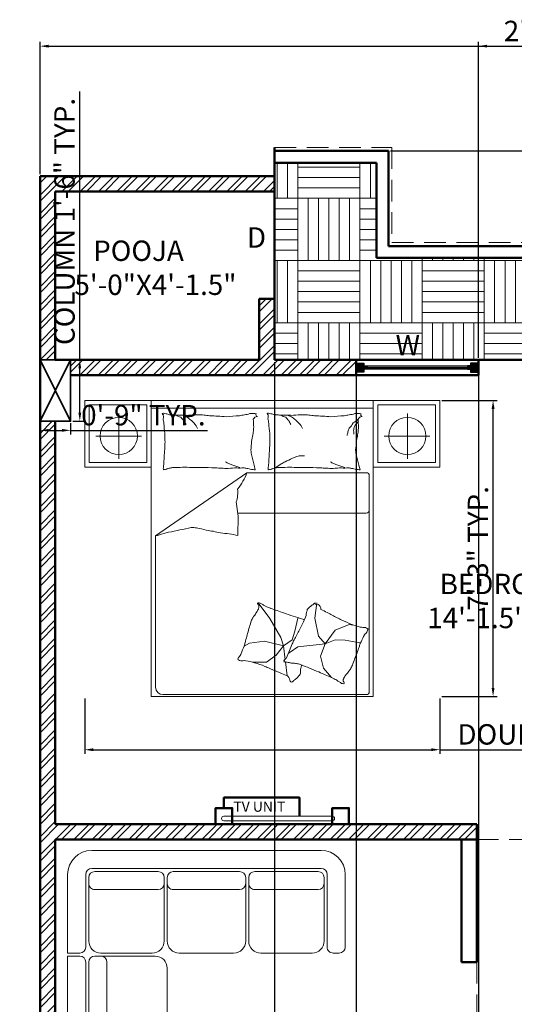
# Model space of a CAD drawing. Units: millimetres. Extents: x 67033 to 68301, y 155969 to 157209.
# Tile 14 of 17: x 67492 to 67638, y 156894 to 157183. Entities that reach past the tile are written whole.
import ezdxf

# ---------------------------------------------------------------- set-up
doc = ezdxf.new("R2010")
doc.units = ezdxf.units.MM
doc.linetypes.add('HIDDEN', pattern=[9.525, 6.35, -3.175])
for name, color, linetype, lineweight in [('A-ANNO-DIMS', 2, 'Continuous', 18), ('A-ANNO-TEXT', 7, 'Continuous', 18), ('A-AREA-IDEN', 3, 'Continuous', 18), ('A-COLS', 3, 'Continuous', 35), ('A-FLOR-OVHD', 1, 'HIDDEN', 18), ('A-FLOR-PATT', 252, 'Continuous', 13), ('A-FURN', 8, 'Continuous', 18), ('A-GLAZ', 4, 'Continuous', 25), ('A-WALL', 7, 'Continuous', 50), ('A-WALL-PATT', 8, 'Continuous', 13)]:
    doc.layers.add(name, color=color, linetype=linetype, lineweight=lineweight)
doc.styles.add('DIM_FONT', font='SIMPLEX.shx', dxfattribs={"width": 0.8})
doc.styles.get("Standard").update_dxf_attribs({"font": 'arial.ttf'})
doc.dimstyles.new('ISO-25', dxfattribs={"dimtxt": 6, "dimasz": 2.5, "dimexe": 1.25, "dimexo": 0.625, "dimtad": 1, "dimdec": 0, "dimlunit": 3, "dimtxsty": 'Standard', "dimcen": 2.5, "dimadec": 0, "dimazin": 0, "dimtfac": 1, "dimtdec": 0, "dimtmove": 0, "dimatfit": 3, "dimfxl": 1, "dimarcsym": 0})
pattern_1 = [(45, (429.8785, 0), (-2.69407684, 2.69407684), []), (45, (431.6745, 0), (-2.69407684, 2.69407684), [])]

# ---------------------------------------------------------------- blocks, each defined once
blk = doc.blocks.new('A$C79766A75')
for p, q in [((0.45, 1.9999), (0, 1.9999)), ((0, 1.9999), (0, 1.5499)), ((0.45, 1.5499), (0.45, 1.9999)), ((1.9506, 2), (0.4506, 2)), ((0.4506, 2), (0.4506, 0)), ((1.9506, 0), (1.9506, 2)), ((2.402, 1.9999), (1.952, 1.9999)), ((1.952, 1.9999), (1.952, 1.5499)), ((2.402, 1.5499), (2.402, 1.9999)), ((0.42, 1.9699), (0.03, 1.9699)), ((0.03, 1.9699), (0.03, 1.5799)), ((0.42, 1.5799), (0.42, 1.9699)), ((1.9506, 1.9476), (0.4506, 1.9476)), ((2.372, 1.9699), (1.982, 1.9699)), ((1.982, 1.9699), (1.982, 1.5799)), ((2.372, 1.5799), (2.372, 1.9699)), ((0.2304, 1.9125), (0.2304, 1.6061)), ((2.1824, 1.9125), (2.1824, 1.6061)), ((0.0743, 1.7595), (0.3834, 1.7595)), ((2.0263, 1.7595), (2.3354, 1.7595)), ((0.4234, 1.6034), (0.4228, 1.6034)), ((1.1461, 1.5617), (1.1254, 1.6443)), ((1.8553, 1.5617), (1.8346, 1.6443)), ((0, 1.5499), (0.45, 1.5499)), ((0.03, 1.5799), (0.42, 1.5799)), ((1.1536, 1.5317), (1.1461, 1.5617)), ((1.8628, 1.5317), (1.8553, 1.5617)), ((1.952, 1.5499), (2.402, 1.5499)), ((1.982, 1.5799), (2.372, 1.5799)), ((1.0972, 1.5115), (0.4791, 1.0841)), ((1.0972, 1.5115), (1.9048, 1.5115)), ((1.9248, 1.4915), (1.9248, 0.0322)), ((1.0383, 1.2184), (1.0246, 1.3138)), ((1.9048, 1.2389), (1.0354, 1.2389)), ((1.0365, 1.0883), (1.0383, 1.2184)), ((0.4791, 0.0622), (0.4791, 1.0841)), ((1.1731, 0.6316), (1.2523, 0.5276)), ((1.5696, 0.6317), (1.5559, 0.5286)), ((1.2523, 0.5276), (1.3274, 0.3973)), ((1.4223, 0.4407), (1.442, 0.5296)), ((1.5559, 0.5286), (1.5817, 0.4065)), ((1.6952, 0.4478), (1.7898, 0.4856)), ((1.7898, 0.4856), (1.8139, 0.4822)), ((1.4025, 0.3834), (1.4223, 0.4407)), ((1.5817, 0.4065), (1.6264, 0.355)), ((1.6264, 0.355), (1.6952, 0.4478)), ((1.1139, 0.3597), (1.0779, 0.3397)), ((1.2167, 0.3736), (1.1139, 0.3597)), ((1.3452, 0.342), (1.2167, 0.3736)), ((1.2957, 0.2787), (1.3452, 0.342)), ((1.3274, 0.3973), (1.3452, 0.342)), ((1.3452, 0.342), (1.4025, 0.3834)), ((1.3452, 0.342), (1.3569, 0.2478)), ((1.4034, 0.3558), (1.3803, 0.2995)), ((1.4406, 0.3361), (1.3907, 0.3)), ((1.6264, 0.355), (1.4406, 0.3361)), ((1.5954, 0.2725), (1.6264, 0.355)), ((1.6264, 0.355), (1.6935, 0.3825)), ((1.6935, 0.3825), (1.7623, 0.379)), ((1.7623, 0.379), (1.8603, 0.3619)), ((1.8603, 0.3619), (1.8636, 0.3554)), ((1.2305, 0.2313), (1.2957, 0.2787)), ((1.3803, 0.2995), (1.3626, 0.256)), ((1.3907, 0.3), (1.3787, 0.2914)), ((1.6161, 0.19), (1.5954, 0.2725)), ((1.1376, 0.2313), (1.2305, 0.2313)), ((1.3588, 0.2331), (1.3706, 0.1385)), ((1.6697, 0.1274), (1.6161, 0.19)), ((1.9048, 0.0122), (0.5291, 0.0122)), ((0.4506, 0), (1.9506, 0))]:
    blk.add_line(p, q)
for centre in [(0.2304, 1.7595), (2.1824, 1.7595)]:
    blk.add_circle(centre, 0.126)
for centre, radius, start, end in [((0.5232, 1.9139), 0.00342, 291.7883, 340.43603), ((0.525, 1.9085), 0.00232, 340.43603, 101.89306), ((0.5246, 1.9378), 0.0251, 274.30254, 291.7883), ((0.5311, 1.9093), 0.00428, 201.9904, 281.89306), ((0.4996, 1.8889), 0.0328, 338.57902, 8.13348), ((0.2896, 1.8253), 0.246, 8.13348, 12.10946), ((0.5465, 1.8994), 0.0156, 158.57902, 201.9904), ((0.5486, 1.9393), 0.0289, 239.34875, 274.30254), ((0.5458, 1.8568), 0.0539, 59.34875, 84.74081), ((0.546, 1.0829), 0.8208, 84.74081, 88.09211), ((0.6118, 2.0005), 0.0992, 254.06476, 274.21588), ((0.6775, 1.9817), 0.0992, 233.91364, 254.06476), ((0.6362, 0.406), 1.4943, 88.09211, 90.57574), ((0.7304, 1.9449), 0.0992, 216.17665, 233.91364), ((0.7737, 2.1075), 0.234, 242.76041, 249.13972), ((0.7661, 1.8961), 0.0992, 198.43965, 216.17665), ((0.7591, 1.0293), 0.8732, 90.57574, 94.80185), ((0.738, 1.949), 0.0768, 231.61143, 242.76041), ((0.974, 2.1633), 0.3916, 226.18849, 231.61143), ((0.7631, 2.1919), 0.2897, 267.46141, 274.80185), ((0.8143, 2.0532), 0.1524, 259.81012, 267.46141), ((0.7515, 1.3747), 0.5293, 79.81012, 83.9133), ((0.8451, 0.8466), 1.049, 83.9133, 90), ((1.046, 1.2129), 0.6827, 90, 97.54685), ((1.1117, 1.6625), 0.2422, 97.54685, 105.74398), ((1.0352, 2.2041), 0.3048, 278.43719, 285.74398), ((1.1179, 2.0719), 0.1611, 270, 278.43719), ((1.171, 1.8579), 0.0342, 94.40021, 153.41948), ((1.6324, 1.8735), 0.4918, 180, 186.23236), ((1.1592, 2.0011), 0.0904, 258.72762, 270), ((1.1709, 1.9049), 0.0131, 153.41948, 258.72762), ((1.2325, 1.9139), 0.00342, 291.7883, 340.43603), ((1.2342, 1.9085), 0.00232, 340.43603, 101.89306), ((1.2338, 1.9378), 0.0251, 274.30254, 291.7883), ((1.2404, 1.9093), 0.00428, 201.9904, 281.89306), ((1.2088, 1.8889), 0.0328, 338.57902, 8.13348), ((0.9988, 1.8253), 0.246, 8.13348, 12.10946), ((1.2558, 1.8994), 0.0156, 158.57902, 201.9904), ((1.2578, 1.9393), 0.0289, 239.34875, 274.30254), ((1.2551, 1.8568), 0.0539, 59.34875, 84.74081), ((1.2552, 1.0829), 0.8208, 84.74081, 88.09211), ((1.3211, 2.0005), 0.0992, 254.06476, 274.21588), ((1.3868, 1.9817), 0.0992, 233.91364, 254.06476), ((1.3455, 0.406), 1.4943, 88.09211, 90.57574), ((1.4396, 1.9449), 0.0992, 216.17665, 233.91364), ((1.4829, 2.1075), 0.234, 242.76041, 249.13972), ((1.4753, 1.8961), 0.0992, 198.43965, 216.17665), ((1.4683, 1.0293), 0.8732, 90.57574, 94.80185), ((1.4473, 1.949), 0.0768, 231.61143, 242.76041), ((1.6833, 2.1633), 0.3916, 226.18849, 231.61143), ((1.4724, 2.1919), 0.2897, 267.46141, 274.80185), ((1.5236, 2.0532), 0.1524, 259.81012, 267.46141), ((1.4607, 1.3747), 0.5293, 79.81012, 83.9133), ((1.5543, 0.8466), 1.049, 83.9133, 90), ((1.7552, 1.2129), 0.6827, 90, 97.54685), ((1.821, 1.6625), 0.2422, 97.54685, 105.74398), ((1.7444, 2.2041), 0.3048, 278.43719, 285.74398), ((1.7511, 1.9723), 0.1399, 297.20359, 314.90238), ((1.8271, 2.0719), 0.1611, 270, 278.43719), ((1.8802, 1.8579), 0.0342, 94.40021, 153.41948), ((2.3416, 1.8735), 0.4918, 180, 186.23236), ((1.8684, 2.0011), 0.0904, 258.72762, 270), ((1.8802, 1.9049), 0.0131, 153.41948, 258.72762), ((0.7297, 1.8867), 0.1983, 187.6809, 192.10946), ((1.4472, 1.8987), 0.9131, 183.36875, 187.6809), ((0.9057, 1.9982), 0.2252, 219.03494, 226.18849), ((0.7932, 1.8591), 0.0493, 208.31676, 219.03494), ((0.9392, 1.9062), 0.2002, 203.00277, 208.31676), ((1.3446, 1.7858), 0.204, 170.31563, 180), ((1.4389, 1.8867), 0.1983, 187.6809, 192.10946), ((2.1565, 1.8987), 0.9131, 183.36875, 187.6809), ((1.615, 1.9982), 0.2252, 219.03494, 226.18849), ((1.5025, 1.8591), 0.0493, 208.31676, 219.03494), ((1.6484, 1.9062), 0.2002, 203.00277, 208.31676), ((1.6554, 1.8529), 0.1399, 332.60117, 343.48502), ((1.6908, 1.9123), 0.1399, 314.90238, 332.60117), ((1.7653, 1.8132), 0.0562, 341.2201, 0), ((1.6307, 1.8895), 0.2056, 338.18508, 341.2201), ((1.6887, 1.8881), 0.1511, 334.64488, 338.18508), ((1.7896, 1.8667), 0.0526, 318.55709, 334.64488), ((1.784, 1.9167), 0.0899, 306.26407, 318.55709), ((2.0538, 1.7858), 0.204, 170.31563, 180), ((1.2208, 1.7573), 0.6787, 178.36691, 183.36875), ((0.8192, 1.792), 0.3171, 347.80162, 351.99495), ((2.0027, 1.5994), 0.882, 167.80162, 170.31563), ((1.9301, 1.7573), 0.6787, 178.36691, 183.36875), ((1.6404, 1.8023), 0.1399, 343.48502, 354.36887), ((1.73, 1.7719), 0.0915, 0, 14.68511), ((1.5284, 1.792), 0.3171, 347.80162, 351.99495), ((2.7119, 1.5994), 0.882, 167.80162, 170.31563), ((14.1519, 0.85), 13.6356, 176.49514, 176.94504), ((1.9066, 1.6447), 1.3652, 176.94504, 178.36691), ((0.4711, 1.7556), 0.6588, 351.99495, 357.33512), ((1.0578, 1.6474), 0.0677, 357.33512, 14.04519), ((14.8612, 0.85), 13.6356, 176.49514, 176.94504), ((2.6158, 1.6447), 1.3652, 176.94504, 178.36691), ((1.1803, 1.7556), 0.6588, 351.99495, 357.33512), ((1.767, 1.6474), 0.0677, 357.33512, 14.04519), ((0.7658, 2.8912), 1.4323, 294.32653, 296.49848), ((1.226, 2.0834), 0.5066, 290.67428, 294.32653), ((1.4305, 1.6796), 0.058, 274.08277, 290.67428), ((1.4679, 1.8969), 0.2721, 266.4448, 274.08277), ((0.8521, 1.5209), 0.3212, 170.00164, 176.49514), ((0.513, 1.535), 0.0193, 350.00164, 16.69777), ((0.5322, 1.5304), 0.00132, 16.69777, 97.12039), ((0.5579, 1.4467), 0.0875, 97.12039, 106.22115), ((0.5822, 1.4654), 0.0767, 106.22115, 117.28412), ((0.5507, 1.5832), 0.0453, 282.86904, 297.28412), ((0.5623, 1.6885), 0.1459, 273.57397, 282.86904), ((0.589, 2.7103), 1.164, 270.28654, 273.57397), ((0.7584, 7.2662), 5.7185, 269.02962, 270.28654), ((0.9401, 4.9065), 3.3622, 267.39037, 269.02962), ((0.9811, 2.7573), 1.2165, 265.38242, 267.39037), ((0.8583, 0.139), 1.4048, 85.38242, 87.25094), ((0.6583, 0.9067), 0.7387, 64.68893, 66.51559), ((1.0175, 1.3138), 0.2301, 87.25094, 101.55856), ((0.7015, 0.888), 0.7387, 66.51559, 68.34226), ((0.7501, 0.8688), 0.7387, 68.34226, 70.57202), ((0.8043, 0.8497), 0.7387, 70.57202, 72.80178), ((1.0449, 1.6886), 0.1459, 263.56595, 281.55856), ((1.1099, 1.6599), 0.1197, 252.61359, 263.56595), ((1.0587, 1.3144), 0.2297, 72.61359, 80.5159), ((1.108, 1.2635), 0.2708, 80.5159, 85.91706), ((1.1535, 1.5308), 0.000917, 85.91706, 194.04494), ((1.5613, 1.5209), 0.3212, 170.00164, 176.49514), ((1.2222, 1.535), 0.0193, 350.00164, 16.69777), ((1.2414, 1.5304), 0.00132, 16.69777, 97.12039), ((1.2671, 1.4467), 0.0875, 97.12039, 106.22115), ((1.2914, 1.4654), 0.0767, 106.22115, 117.28412), ((1.2599, 1.5832), 0.0453, 282.86904, 297.28412), ((1.2716, 1.6885), 0.1459, 273.57397, 282.86904), ((0.9025, 2.1618), 0.7286, 302.13498, 305.82629), ((1.2982, 2.7103), 1.164, 270.28654, 273.57397), ((1.1895, 1.8508), 0.3126, 296.49848, 302.13498), ((1.4677, 7.2662), 5.7185, 269.02962, 270.28654), ((1.6493, 4.9065), 3.3622, 267.39037, 269.02962), ((1.6903, 2.7573), 1.2165, 265.38242, 267.39037), ((1.5676, 0.139), 1.4048, 85.38242, 87.25094), ((1.3675, 0.9067), 0.7387, 64.68893, 66.51559), ((1.7268, 1.3138), 0.2301, 87.25094, 101.55856), ((1.4107, 0.888), 0.7387, 66.51559, 68.34226), ((1.4594, 0.8688), 0.7387, 68.34226, 70.57202), ((1.5136, 0.8497), 0.7387, 70.57202, 72.80178), ((1.7541, 1.6886), 0.1459, 263.56595, 281.55856), ((1.8192, 1.6599), 0.1197, 252.61359, 263.56595), ((1.7679, 1.3144), 0.2297, 72.61359, 80.5159), ((1.8172, 1.2635), 0.2708, 80.5159, 85.91706), ((1.8627, 1.5308), 0.000917, 85.91706, 194.04494), ((0.745, 1.6407), 0.3751, 320.35546, 339.85116), ((1.9048, 1.4915), 0.02, 0, 90), ((0.8556, 1.3759), 0.1801, 339.85116, 8.13558), ((1.9048, 1.2589), 0.02, 270, 0), ((-0.1888, 5.1029), 4.0646, 280.72756, 282.92554), ((0.7282, 1.1989), 0.0581, 262.26962, 280.72756), ((0.7833, 1.3309), 0.1942, 256.8096, 262.26962), ((0.2481, -1.3253), 2.5158, 76.8096, 78.32586), ((-0.0248, 2.8487), 1.8351, 285.93519, 287.73639), ((0.3872, 1.7415), 0.6574, 282.92554, 285.93519), ((0.3953, -1.4284), 2.588, 78.32586, 80.50498), ((0.413, -2.64), 3.7801, 80.50498, 82.308), ((1.1752, 0.6267), 0.0063, 166.71916, 233.42082), ((1.1734, 0.6272), 0.00443, 93.94836, 166.71916), ((1.163, 0.6103), 0.0142, 10.40739, 53.42082), ((1.1755, 0.5964), 0.0352, 69.65479, 93.94836), ((1.1011, 0.5989), 0.0771, 2.72862, 10.40739), ((1.1628, 0.6019), 0.0153, 345.42909, 2.72862), ((1.1669, 0.5731), 0.0601, 51.41461, 69.65479), ((1.2538, 0.682), 0.0792, 231.41461, 247.29308), ((1.5463, 1.3811), 0.8371, 247.29308, 249.87133), ((1.383, 0.7705), 0.2176, 307.21509, 313.52244), ((1.1426, 1.1456), 0.6605, 306.2163, 307.21509), ((1.7751, 0.3162), 0.3825, 126.2163, 127.52874), ((1.5806, 0.5924), 0.0452, 127.52874, 134.1274), ((1.5093, 0.6825), 0.0697, 308.81361, 314.1274), ((1.5706, 0.6318), 0.0127, 176.75451, 308.81361), ((1.5621, 0.59), 0.0359, 356.75451, 62.70976), ((1.2077, 0.4922), 0.081, 140.29953, 153.92651), ((0.9961, 0.6678), 0.194, 320.29953, 329.09437), ((0.8605, 0.749), 0.352, 329.09437, 333.18207), ((1.1396, 0.6079), 0.0393, 333.18207, 345.42909), ((3.0113, 5.3783), 5.0942, 249.87133, 250.91638), ((2.374, 3.5362), 3.145, 250.91638, 253.39153), ((2.4089, 0.1204), 1.0054, 154.94715, 157.58378), ((1.5435, 0.5526), 0.0458, 157.58378, 188.04918), ((1.4828, 0.5833), 0.0226, 324.10643, 8.04918), ((1.4519, 0.6426), 0.0774, 313.52244, 324.10643), ((0.2201, -2.1858), 3.0972, 62.70976, 63.58535), ((2.5711, 2.3551), 2.0162, 242.50014, 243.58535), ((4.5245, 5.9445), 6.1019, 242.15178, 242.50014), ((3.0311, -0.112), 2.003, 162.1604, 164.73746), ((1.3115, 0.4414), 0.1965, 153.92651, 162.1604), ((2.9813, -0.2643), 1.6868, 152.91165, 154.94715), ((1.5084, 0.6341), 0.1166, 253.39153, 259.26338), ((-0.9881, -4.647), 5.8383, 62.15178, 62.50792), ((1.5182, -0.068), 0.6236, 62.50792, 69.25137), ((1.7121, 0.0657), 0.43, 69.25137, 77.37478), ((1.8682, 0.4049), 0.063, 77.37478, 93.38812), ((1.8955, 0.5247), 0.0599, 256.95977, 273.38812), ((2.6887, -0.0186), 1.6481, 164.73746, 166.159), ((2.8096, -0.3311), 1.5652, 150.06403, 152.91165), ((-0.5166, 1.5491), 2.6619, 333.66682, 334.82685), ((1.8435, 0.4743), 0.0755, 310.50865, 333.66682), ((1.9257, 0.5082), 0.0509, 238.30826, 256.95977), ((1.9279, 0.441), 0.0168, 130.50865, 180.96136), ((1.9201, 0.4587), 0.0058, 180.96136, 238.30826), ((-1.4109, 1.284), 2.6619, 338.0627, 339.22273), ((0.9098, 0.4035), 0.1798, 339.22273, 343.68776), ((0.5589, 0.5062), 0.5454, 343.68776, 346.159), ((1.2176, 0.4627), 0.2143, 330.06403, 337.76452), ((3.4079, -0.2212), 1.6481, 160.34158, 161.76311), ((1.3456, 0.5261), 0.5454, 339.29188, 341.76311), ((1.701, 0.4319), 0.1798, 334.82685, 339.29188), ((0.9882, 0.3177), 0.0755, 314.90453, 338.0627), ((3.6966, -0.4634), 2.003, 157.76452, 160.34158), ((1.0533, 0.2524), 0.0168, 134.90453, 185.35724), ((1.0424, 0.2513), 0.0058, 185.35724, 242.70414), ((1.0631, 0.2914), 0.0509, 242.70414, 261.35565), ((1.0645, 0.3003), 0.0599, 261.35565, 277.784), ((1.0811, 0.1786), 0.063, 81.77066, 97.784), ((1.0286, -0.1846), 0.43, 73.64725, 81.77066), ((0.974, -0.3705), 0.6236, 66.9038, 73.64725), ((-1.0716, -5.1672), 5.8383, 66.54766, 66.9038), ((1.3465, 0.2383), 0.00467, 287.18674, 70.62007), ((1.3486, 0.2247), 0.0092, 70.62007, 94.25932), ((1.3694, 0.234), 0.0231, 107.18674, 157.76452), ((1.3563, 0.267), 0.034, 262.01776, 274.25932), ((1.4091, 0.4221), 0.1955, 255.1193, 262.01776), ((1.358, 0.0507), 0.1794, 75.1193, 82.32164), ((1.4096, 0.153), 0.0712, 82.32164, 94.51184), ((1.4285, 0.2893), 0.0663, 261.87843, 274.51184), ((1.4755, 0.332), 0.1166, 248.99565, 261.87843), ((2.7121, 3.1012), 3.145, 246.5205, 248.99565), ((2.4175, -0.1202), 1.0054, 160.65521, 161.97966), ((1.9797, 0.1108), 0.1965, 149.53063, 157.76452), ((3.6805, 5.7866), 6.1019, 246.54766, 246.89602), ((2.0773, 2.0287), 2.0162, 246.89602, 247.98123), ((0.1602, -2.7118), 3.0972, 67.10564, 67.98123), ((1.3512, 0.1084), 0.0359, 1.15039, 67.10564), ((1.2874, 0.2845), 0.2176, 311.61098, 317.91833), ((1.3914, 0.1905), 0.0774, 317.91833, 328.50231), ((1.4382, 0.1619), 0.0226, 328.50231, 12.44506), ((1.505, 0.1766), 0.0458, 161.97966, 192.44506), ((3.6993, 4.7998), 5.0942, 245.47545, 246.5205), ((1.4661, 0.3294), 0.352, 324.69849, 328.78619), ((1.6279, 0.2819), 0.194, 315.90365, 324.69849), ((1.856, 0.1288), 0.081, 135.90365, 149.53063), ((1.3997, 0.1094), 0.0127, 181.15039, 313.2095), ((1.3607, 0.1509), 0.0697, 313.2095, 318.52329), ((1.4468, 0.0748), 0.0452, 131.92462, 138.52329), ((1.6722, -0.1762), 0.3825, 130.61218, 131.92462), ((0.9933, 0.6156), 0.6605, 310.61218, 311.61098), ((2.051, 0.8725), 0.8371, 242.8972, 245.47545), ((1.7576, 0.1689), 0.0792, 227.01873, 242.8972), ((1.6963, 0.0438), 0.0601, 47.01873, 65.25891), ((1.737, 0.0526), 0.0352, 65.25891, 89.55248), ((1.7345, 0.1188), 0.0153, 341.03321, 358.33274), ((1.6723, 0.1058), 0.0771, 358.33274, 6.01151), ((1.7401, 0.0928), 0.0142, 6.01151, 49.02494), ((1.7162, 0.1388), 0.0393, 328.78619, 341.03321), ((1.756, 0.0832), 0.00443, 89.55248, 162.32327), ((1.7602, 0.0924), 0.0063, 162.32327, 229.02494), ((0.5291, 0.0622), 0.05, 180, 270), ((1.9048, 0.0322), 0.02, 270, 0)]:
    blk.add_arc(centre, radius, start, end)
at = {"style": 'DIM_FONT', "text_generation_flag": 4, "width": 0.8, "flags": 9}
for tag in ['XSIZE', 'YSIZE']:
    blk.add_attdef(tag, (1.9506, 2), '', height=0.0005, rotation=180, dxfattribs=at)
blk = doc.blocks.new('A$C2AFA021D')
for p, q in [((0.8, 2.3), (0.2, 2.3)), ((0.85, 2.2), (0.85, 2.25)), ((0.2, 2.15), (0.8, 2.15)), ((0.225, 2.125), (0.275, 2.125)), ((0.75, 2.125), (0.275, 2.125)), ((0, 2.1), (0, 0.2)), ((0.15, 0.2), (0.15, 2.1)), ((0.175, 1.55), (0.175, 2.075)), ((0.325, 2.075), (0.325, 1.55)), ((0.85, 1.6), (0.85, 2.025)), ((0.275, 1.5), (0.225, 1.5)), ((0.225, 1.475), (0.275, 1.475)), ((0.275, 1.5), (0.75, 1.5)), ((0.75, 1.475), (0.275, 1.475)), ((0.175, 0.875), (0.175, 1.425)), ((0.325, 1.425), (0.325, 0.875)), ((0.85, 0.925), (0.85, 1.375)), ((0.275, 0.825), (0.225, 0.825)), ((0.275, 0.825), (0.75, 0.825)), ((0.975, 0.825), (1.4, 0.825)), ((1.625, 0.825), (2.075, 0.825)), ((2.3, 0.825), (2.725, 0.825)), ((2.9, 0.825), (2.95, 0.825)), ((0.175, 0.225), (0.175, 0.75)), ((0.225, 0.8), (0.275, 0.8)), ((0.75, 0.8), (0.275, 0.8)), ((0.325, 0.75), (0.325, 0.225)), ((2.85, 0.2), (2.85, 0.775)), ((3, 0.775), (3, 0.2)), ((0.85, 0.275), (0.85, 0.7)), ((0.875, 0.275), (0.875, 0.725)), ((1.5, 0.725), (1.5, 0.275)), ((1.525, 0.275), (1.525, 0.725)), ((2.175, 0.725), (2.175, 0.275)), ((2.2, 0.275), (2.2, 0.725)), ((2.825, 0.725), (2.825, 0.275)), ((0.875, 0.275), (0.875, 0.225)), ((1.45, 0.325), (0.925, 0.325)), ((1.5, 0.225), (1.5, 0.275)), ((1.525, 0.275), (1.525, 0.225)), ((2.125, 0.325), (1.575, 0.325)), ((2.175, 0.225), (2.175, 0.275)), ((2.2, 0.275), (2.2, 0.225)), ((2.775, 0.325), (2.25, 0.325)), ((2.825, 0.225), (2.825, 0.275)), ((0.275, 0.175), (0.225, 0.175)), ((0.275, 0.175), (0.75, 0.175)), ((0.925, 0.175), (1.45, 0.175)), ((1.575, 0.175), (2.125, 0.175)), ((2.25, 0.175), (2.775, 0.175)), ((0.8, 0.15), (0.2, 0.15)), ((0.85, 0), (0.85, 0.1)), ((0.875, 0.1), (0.875, 0)), ((0.925, 0.15), (2.8, 0.15)), ((0.2, 0), (0.85, 0)), ((2.8, 0), (0.875, 0))]:
    blk.add_line(p, q)
for centre, radius, start, end in [((0.2, 2.1), 0.2, 90, 180), ((0.8, 2.25), 0.05, 0, 90), ((0.2, 2.1), 0.05, 90, 180), ((0.225, 2.075), 0.05, 90, 180), ((0.275, 2.075), 0.05, 0, 90), ((0.75, 2.025), 0.1, 0, 90), ((0.8, 2.2), 0.05, 270, 0), ((0.225, 1.55), 0.05, 180, 270), ((0.275, 1.55), 0.05, 270, 0), ((0.75, 1.6), 0.1, 270, 0), ((0.225, 1.425), 0.05, 90, 180), ((0.275, 1.425), 0.05, 0, 90), ((0.75, 1.375), 0.1, 360, 90), ((0.75, 0.925), 0.1, 270, 0), ((0.225, 0.875), 0.05, 180, 270), ((0.275, 0.875), 0.05, 270, 0), ((0.975, 0.725), 0.1, 90, 180), ((1.4, 0.725), 0.1, 0, 90), ((1.625, 0.725), 0.1, 90, 180), ((2.075, 0.725), 0.1, 0, 90), ((2.3, 0.725), 0.1, 90, 180), ((2.725, 0.725), 0.1, 0, 90), ((2.9, 0.775), 0.05, 90, 180), ((2.95, 0.775), 0.05, 0, 90), ((0.225, 0.75), 0.05, 90, 180), ((0.275, 0.75), 0.05, 0, 90), ((0.75, 0.7), 0.1, 0, 90), ((0.75, 0.275), 0.1, 270, 0), ((0.925, 0.275), 0.05, 90, 180), ((1.45, 0.275), 0.05, 360, 90), ((1.575, 0.275), 0.05, 90, 180), ((2.125, 0.275), 0.05, 360, 90), ((2.25, 0.275), 0.05, 90, 180), ((2.775, 0.275), 0.05, 360, 90), ((0.2, 0.2), 0.2, 180, 270), ((0.2, 0.2), 0.05, 180, 270), ((0.225, 0.225), 0.05, 180, 270), ((0.275, 0.225), 0.05, 270, 0), ((0.925, 0.225), 0.05, 180, 270), ((1.45, 0.225), 0.05, 270, 0), ((1.575, 0.225), 0.05, 180, 270), ((2.125, 0.225), 0.05, 270, 0), ((2.25, 0.225), 0.05, 180, 270), ((2.775, 0.225), 0.05, 270, 0), ((2.8, 0.2), 0.2, 270, 0), ((2.8, 0.2), 0.05, 270, 0), ((0.8, 0.1), 0.05, 0, 90), ((0.925, 0.1), 0.05, 90, 180)]:
    blk.add_arc(centre, radius, start, end)
blk = doc.blocks.new('WIN-900')
for p, q in [((3.67, 3.22), (33.2, 3.22)), ((3.67, 2.74), (33.2, 2.74)), ((33.2, 2.27), (3.67, 2.27))]:
    blk.add_line(p, q)
blk.add_lwpolyline([(0.44, 4.99), (36.44, 4.99), (36.44, 0.49), (0.44, 0.49)], close=True)
for points in [[(0.44, 4.09), (2.73, 4.09), (2.73, 3.22), (3.67, 3.22), (3.67, 2.27), (2.73, 2.27), (2.73, 1.4), (0.44, 1.4)], [(36.44, 4.09), (34.14, 4.09), (34.14, 3.22), (33.2, 3.22), (33.2, 2.27), (34.14, 2.27), (34.14, 1.4), (36.44, 1.4)]]:
    blk.add_lwpolyline(points)
blk = doc.blocks.new('COLUMN-230x460')
for p, q in [((0.44, 17.99), (9.44, -0.01)), ((9.44, 17.99), (0.44, -0.01))]:
    blk.add_line(p, q)
blk.add_lwpolyline([(0.44, 17.99), (9.44, 17.99), (9.44, -0.01), (0.44, -0.01)], close=True)
blk = doc.blocks.new('TV-UNIT')
for points in [[(0.68, 1.36), (32.57, 1.36)], [(32.57, 0), (0.68, 0)]]:
    blk.add_lwpolyline(points)
for centre, start, end in [((0.68, 0.68), 90, 270), ((32.57, 0.68), 270, 90)]:
    blk.add_arc(centre, 0.678, start, end)
blk = doc.blocks.new('*D49')
at = {"layer": 'A-ANNO-DIMS', "color": 0, "lineweight": -2, "transparency": 16777216}
for p, q in [((67510.02, 157082.99), (67510.02, 157161.9)), ((67507.94, 157082.99), (67511.27, 157082.99)), ((67510.02, 157067.49), (67510.02, 157080.49)), ((67507.94, 157064.99), (67511.27, 157064.99))]:
    blk.add_line(p, q, dxfattribs=at)
at = {"layer": 'A-ANNO-DIMS', "color": 0, "transparency": 16777216}
for points in [[(67509.6, 157080.49), (67510.43, 157080.49), (67510.02, 157082.99)], [(67509.6, 157067.49), (67510.43, 157067.49), (67510.02, 157064.99)]]:
    blk.add_solid(points, dxfattribs=at)
at = {"layer": 'Defpoints', "color": 0, "transparency": 16777216}
for p in [(67507.32, 157082.99), (67510.02, 157082.99), (67507.32, 157064.99)]:
    blk.add_point(p, dxfattribs=at)
at = {"layer": 'A-ANNO-DIMS', "color": 0, "transparency": 16777216, "insert": (67506.29, 157123.7), "char_height": 6, "attachment_point": 5, "rotation": 90}
blk.add_mtext('COLUMN 1\'-6" TYP.', dxfattribs=at)
blk = doc.blocks.new('*D50')
at = {"layer": 'A-ANNO-DIMS', "color": 0, "lineweight": -2, "transparency": 16777216}
for p, q in [((67498.32, 157064.37), (67498.32, 157061.04)), ((67507.32, 157064.37), (67507.32, 157061.04)), ((67500.82, 157062.29), (67504.82, 157062.29)), ((67507.32, 157062.29), (67547.64, 157062.29))]:
    blk.add_line(p, q, dxfattribs=at)
at = {"layer": 'A-ANNO-DIMS', "color": 0, "transparency": 16777216}
for points in [[(67500.82, 157062.71), (67500.82, 157061.88), (67498.32, 157062.29)], [(67504.82, 157062.71), (67504.82, 157061.88), (67507.32, 157062.29)]]:
    blk.add_solid(points, dxfattribs=at)
at = {"layer": 'Defpoints', "color": 0, "transparency": 16777216}
for p in [(67498.32, 157064.99), (67507.32, 157064.99), (67507.32, 157062.29)]:
    blk.add_point(p, dxfattribs=at)
at = {"layer": 'A-ANNO-DIMS', "color": 0, "transparency": 16777216, "insert": (67528.73, 157065.98), "char_height": 6, "attachment_point": 5}
blk.add_mtext('0\'-9" TYP.', dxfattribs=at)
blk = doc.blocks.new('*D55')
at = {"layer": 'A-ANNO-DIMS', "color": 0, "lineweight": -2, "transparency": 16777216}
for p, q in [((67511.46, 156983.46), (67511.46, 156967.16)), ((67615.96, 156983.46), (67615.96, 156967.16)), ((67513.96, 156968.41), (67613.46, 156968.41)), ((67615.96, 156968.41), (67726.32, 156968.41))]:
    blk.add_line(p, q, dxfattribs=at)
at = {"layer": 'A-ANNO-DIMS', "color": 0, "transparency": 16777216}
for points in [[(67513.96, 156968.83), (67513.96, 156967.99), (67511.46, 156968.41)], [(67613.46, 156968.83), (67613.46, 156967.99), (67615.96, 156968.41)]]:
    blk.add_solid(points, dxfattribs=at)
at = {"layer": 'Defpoints', "color": 0, "transparency": 16777216}
for p in [(67511.46, 156984.08), (67615.96, 156984.08), (67615.96, 156968.41)]:
    blk.add_point(p, dxfattribs=at)
at = {"layer": 'A-ANNO-DIMS', "color": 0, "transparency": 16777216, "insert": (67672.39, 156972.14), "char_height": 6, "attachment_point": 5}
blk.add_mtext('DOUBLE BED 8\'-8 1/2" TYP.', dxfattribs=at)
blk = doc.blocks.new('*D56')
at = {"layer": 'A-ANNO-DIMS', "color": 0, "lineweight": -2, "transparency": 16777216}
for p, q in [((67616.58, 157071.11), (67632.88, 157071.11)), ((67631.63, 156986.58), (67631.63, 157068.61)), ((67616.58, 156984.08), (67632.88, 156984.08))]:
    blk.add_line(p, q, dxfattribs=at)
at = {"layer": 'A-ANNO-DIMS', "color": 0, "transparency": 16777216}
for points in [[(67631.21, 157068.61), (67632.05, 157068.61), (67631.63, 157071.11)], [(67631.21, 156986.58), (67632.05, 156986.58), (67631.63, 156984.08)]]:
    blk.add_solid(points, dxfattribs=at)
at = {"layer": 'Defpoints', "color": 0, "transparency": 16777216}
for p in [(67615.96, 157071.11), (67631.63, 157071.11), (67615.96, 156984.08)]:
    blk.add_point(p, dxfattribs=at)
at = {"layer": 'A-ANNO-DIMS', "color": 0, "transparency": 16777216, "insert": (67627.94, 157027.6), "char_height": 6, "attachment_point": 5, "rotation": 90}
blk.add_mtext('7\'-3" TYP.', dxfattribs=at)
blk = doc.blocks.new('*D96')
at = {"layer": 'A-ANNO-DIMS', "color": 0, "lineweight": -2, "transparency": 16777216}
for p, q in [((67567.32, 157082.37), (67567.32, 156531.49)), ((67591.32, 157082.37), (67591.32, 156531.49)), ((67569.82, 156532.74), (67588.82, 156532.74))]:
    blk.add_line(p, q, dxfattribs=at)
at = {"layer": 'A-ANNO-DIMS', "color": 0, "transparency": 16777216}
for points in [[(67569.82, 156533.16), (67569.82, 156532.33), (67567.32, 156532.74)], [(67588.82, 156533.16), (67588.82, 156532.33), (67591.32, 156532.74)]]:
    blk.add_solid(points, dxfattribs=at)
at = {"layer": 'Defpoints', "color": 0, "transparency": 16777216}
for p in [(67567.32, 157082.99), (67591.32, 157082.99), (67591.32, 156532.74)]:
    blk.add_point(p, dxfattribs=at)
at = {"layer": 'A-ANNO-DIMS', "color": 0, "transparency": 16777216, "insert": (67579.32, 156536.43), "char_height": 6, "attachment_point": 5}
blk.add_mtext('2\'-0"', dxfattribs=at)
blk = doc.blocks.new('*D97')
at = {"layer": 'A-ANNO-DIMS', "color": 0, "lineweight": -2, "transparency": 16777216}
for p, q in [((67591.32, 157082.37), (67591.32, 156531.49)), ((67627.32, 157082.37), (67627.32, 156531.49)), ((67593.82, 156532.74), (67624.82, 156532.74))]:
    blk.add_line(p, q, dxfattribs=at)
at = {"layer": 'A-ANNO-DIMS', "color": 0, "transparency": 16777216}
for points in [[(67593.82, 156533.16), (67593.82, 156532.33), (67591.32, 156532.74)], [(67624.82, 156533.16), (67624.82, 156532.33), (67627.32, 156532.74)]]:
    blk.add_solid(points, dxfattribs=at)
at = {"layer": 'Defpoints', "color": 0, "transparency": 16777216}
for p in [(67591.32, 157082.99), (67627.32, 157082.99), (67627.32, 156532.74)]:
    blk.add_point(p, dxfattribs=at)
at = {"layer": 'A-ANNO-DIMS', "color": 0, "transparency": 16777216, "insert": (67609.32, 156536.43), "char_height": 6, "attachment_point": 5}
blk.add_mtext('3\'-0"', dxfattribs=at)
blk = doc.blocks.new('*D98')
at = {"layer": 'A-ANNO-DIMS', "color": 0, "lineweight": -2, "transparency": 16777216}
for p, q in [((67627.32, 157083.62), (67627.32, 157176.49)), ((67629.82, 157175.24), (67657.82, 157175.24)), ((67660.32, 157083.62), (67660.32, 157176.49))]:
    blk.add_line(p, q, dxfattribs=at)
at = {"layer": 'A-ANNO-DIMS', "color": 0, "transparency": 16777216}
for points in [[(67629.82, 157175.66), (67629.82, 157174.83), (67627.32, 157175.24)], [(67657.82, 157175.66), (67657.82, 157174.83), (67660.32, 157175.24)]]:
    blk.add_solid(points, dxfattribs=at)
at = {"layer": 'Defpoints', "color": 0, "transparency": 16777216}
for p in [(67660.32, 157175.24), (67627.32, 157082.99), (67660.32, 157082.99)]:
    blk.add_point(p, dxfattribs=at)
at = {"layer": 'A-ANNO-DIMS', "color": 0, "transparency": 16777216, "insert": (67643.82, 157178.93), "char_height": 6, "attachment_point": 5}
blk.add_mtext('2\'-9"', dxfattribs=at)
blk = doc.blocks.new('*D111')
at = {"layer": 'A-ANNO-DIMS', "color": 0, "lineweight": -2, "transparency": 16777216}
for p, q in [((67498.32, 157137.62), (67498.32, 157176.49)), ((67500.82, 157175.24), (67834.82, 157175.24)), ((67837.32, 157083.62), (67837.32, 157176.49))]:
    blk.add_line(p, q, dxfattribs=at)
at = {"layer": 'A-ANNO-DIMS', "color": 0, "transparency": 16777216}
for points in [[(67500.82, 157175.66), (67500.82, 157174.83), (67498.32, 157175.24)], [(67834.82, 157175.66), (67834.82, 157174.83), (67837.32, 157175.24)]]:
    blk.add_solid(points, dxfattribs=at)
at = {"layer": 'Defpoints', "color": 0, "transparency": 16777216}
for p in [(67837.32, 157175.24), (67498.32, 157136.99), (67837.32, 157082.99)]:
    blk.add_point(p, dxfattribs=at)
at = {"layer": 'A-ANNO-DIMS', "color": 0, "transparency": 16777216, "insert": (67667.82, 157178.93), "char_height": 6, "attachment_point": 5}
blk.add_mtext('28\'-3"', dxfattribs=at)
blk = doc.blocks.new('*D112')
at = {"layer": 'A-ANNO-DIMS', "color": 0, "lineweight": -2, "transparency": 16777216}
for p, q in [((67601.44, 157144.49), (67868.32, 157144.49)), ((67867.07, 157141.99), (67867.07, 156564.99)), ((67768.94, 156562.49), (67868.32, 156562.49))]:
    blk.add_line(p, q, dxfattribs=at)
at = {"layer": 'A-ANNO-DIMS', "color": 0, "transparency": 16777216}
for points in [[(67866.65, 157141.99), (67867.48, 157141.99), (67867.07, 157144.49)], [(67866.65, 156564.99), (67867.48, 156564.99), (67867.07, 156562.49)]]:
    blk.add_solid(points, dxfattribs=at)
at = {"layer": 'Defpoints', "color": 0, "transparency": 16777216}
for p in [(67600.82, 157144.49), (67768.32, 156562.49), (67867.07, 156562.49)]:
    blk.add_point(p, dxfattribs=at)
at = {"layer": 'A-ANNO-DIMS', "color": 0, "transparency": 16777216, "insert": (67863.38, 156853.49), "char_height": 6, "attachment_point": 5, "rotation": 90}
blk.add_mtext('48\'-6"', dxfattribs=at)

msp = doc.modelspace()

# ---------------------------------------------------------------- hatches: boundary and pattern name
at = {"layer": 'A-FLOR-PATT'}
h = msp.add_hatch(dxfattribs=at)
h.set_pattern_fill('AR-PARQ1', color=256, scale=0.06)
h.paths.add_polyline_path([(67832.82, 157112.99), (67597.32, 157112.99), (67597.32, 157140.99), (67567.32, 157140.99), (67567.32, 157082.99), (67627.32, 157082.99), (67660.32, 157082.99), (67832.82, 157082.99)])
h.paths.add_polyline_path([(67595.94, 157081.09), (67613.84, 157081.09), (67613.84, 157093.46), (67595.94, 157093.46)], flags=9)
h.paths.add_polyline_path([(67740.95, 157081.83), (67758.84, 157081.83), (67758.84, 157094.2), (67740.95, 157094.2)], flags=9)
at = {"layer": 'A-GLAZ'}
h = msp.add_hatch(color=256, dxfattribs=at)
h.dxf.hatch_style = 1
h.paths.add_polyline_path([(67594.55, 157081.22), (67593.61, 157081.22), (67593.61, 157082.09), (67591.32, 157082.09), (67591.32, 157079.4), (67593.61, 157079.4), (67593.61, 157080.27), (67594.55, 157080.27)])
h = msp.add_hatch(color=256, dxfattribs=at)
h.dxf.hatch_style = 1
h.paths.add_polyline_path([(67627.32, 157082.09), (67625.02, 157082.09), (67625.02, 157081.22), (67624.08, 157081.22), (67624.08, 157080.27), (67625.02, 157080.27), (67625.02, 157079.4), (67627.32, 157079.4)])
at = {"layer": 'A-WALL-PATT'}
h = msp.add_hatch(dxfattribs=at)
h.set_pattern_fill('ANSI32', color=256, scale=0.4)
h.set_pattern_definition(pattern_1)
h.paths.add_polyline_path([(67502.82, 157132.49), (67567.32, 157132.49), (67567.32, 157136.99), (67498.32, 157136.99), (67498.32, 157082.99), (67502.82, 157082.99)])
h = msp.add_hatch(dxfattribs=at)
h.set_pattern_fill('ANSI32', color=256, scale=0.4)
h.set_pattern_definition(pattern_1)
h.paths.add_polyline_path([(67591.32, 157082.99), (67567.32, 157082.99), (67567.32, 157100.99), (67562.82, 157100.99), (67562.82, 157082.99), (67507.32, 157082.99), (67507.32, 157078.49), (67591.32, 157078.49)])
h = msp.add_hatch(dxfattribs=at)
h.set_pattern_fill('ANSI32', color=256, scale=0.4)
h.set_pattern_definition(pattern_1)
h.paths.add_polyline_path([(67502.82, 157064.99), (67498.32, 157064.99), (67498.32, 156835.49), (67502.82, 156835.49), (67502.82, 156941.99), (67626.86, 156941.99), (67626.86, 156946.49), (67502.82, 156946.49)])

# ---------------------------------------------------------------- linework, layer by layer
at = {"layer": 'A-FLOR-OVHD'}
for p, q in [((67567.32, 157145.49), (67601.82, 157145.49)), ((67601.82, 157145.49), (67601.82, 157117.49)), ((67601.82, 157117.49), (67837.32, 157117.49)), ((67626.86, 156941.99), (67660.32, 156941.99)), ((67626.86, 156905.99), (67626.86, 156821.99))]:
    msp.add_line(p, q, dxfattribs=at)
at = {"layer": 'A-WALL'}
for p, q in [((67567.32, 157145.49), (67567.32, 157082.99)), ((67567.32, 157144.49), (67600.82, 157144.49)), ((67600.82, 157144.49), (67600.82, 157116.49)), ((67567.32, 157140.99), (67597.32, 157140.99)), ((67597.32, 157140.99), (67597.32, 157112.99)), ((67498.32, 157136.99), (67498.32, 156622.48)), ((67567.32, 157136.99), (67498.32, 157136.99)), ((67502.82, 157132.49), (67502.82, 157082.99)), ((67502.82, 157132.49), (67567.32, 157132.49)), ((67600.82, 157116.49), (67836.32, 157116.49)), ((67597.32, 157112.99), (67832.82, 157112.99)), ((67562.82, 157100.99), (67562.82, 157082.99)), ((67562.82, 157100.99), (67567.32, 157100.99)), ((67502.82, 157082.99), (67562.82, 157082.99)), ((67567.32, 157082.99), (67627.32, 157082.99)), ((67591.32, 157082.99), (67591.32, 157078.49)), ((67627.32, 157082.99), (67627.32, 157078.49)), ((67627.32, 157082.99), (67660.32, 157082.99)), ((67507.32, 157078.49), (67627.32, 157078.49)), ((67502.82, 157064.99), (67502.82, 156946.49)), ((67502.82, 156946.49), (67626.86, 156946.49)), ((67626.86, 156946.49), (67626.86, 156905.99)), ((67502.82, 156941.99), (67502.82, 156835.49)), ((67502.82, 156941.99), (67626.86, 156941.99)), ((67622.36, 156941.99), (67622.36, 156905.99)), ((67622.36, 156905.99), (67626.86, 156905.99))]:
    msp.add_line(p, q, dxfattribs=at)
msp.add_lwpolyline([(67552.41, 156951.23), (67552.41, 156954.35), (67574.66, 156954.35), (67574.66, 156948.86)], dxfattribs=at)
for points in [[(67549.96, 156946.49), (67554.87, 156946.49), (67554.87, 156951.23), (67549.96, 156951.23)], [(67584.3, 156946.49), (67589.21, 156946.49), (67589.21, 156951.23), (67584.3, 156951.23)]]:
    msp.add_lwpolyline(points, close=True, dxfattribs=at)

# ---------------------------------------------------------------- block references
at = {"layer": 'A-COLS'}
msp.add_blockref('COLUMN-230x460', (67497.88, 157065), dxfattribs=at)
at = {"layer": 'A-FURN', "xscale": 43.50257579484658, "yscale": 43.50257579484658, "zscale": 43.50257579484658}
msp.add_blockref('A$C79766A75', (67511.46, 156984.08), dxfattribs=at)
at = {"layer": 'A-FURN', "rotation": 180}
msp.add_blockref('TV-UNIT', (67584.98, 156948.86), dxfattribs=at)
at = {"layer": 'A-FURN', "xscale": 35.51344104378158, "yscale": 35.51344104378158, "zscale": 35.51344104378158, "rotation": 270}
msp.add_blockref('A$C2AFA021D', (67506.45, 156938.81), dxfattribs=at)
at = {"layer": 'A-GLAZ'}
msp.add_blockref('WIN-900', (67590.88, 157078), dxfattribs=at)

# ---------------------------------------------------------------- texts
at = {"layer": 'A-ANNO-TEXT', "attachment_point": 1}
for s, width, insert, char_height in [('   D', 19.5287, (67553.69, 157121.99), 6), ('   W', 19.5287, (67597.44, 157090.37), 6), ('  TV UNIT', 25.6344, (67553.38, 156953.18), 3)]:
    msp.add_mtext_dynamic_manual_height_columns(s, width=width, gutter_width=12.5, heights=[0], dxfattribs=dict(at, insert=insert, char_height=char_height))
at = {"layer": 'A-AREA-IDEN', "char_height": 6, "attachment_point": 1}
for s, insert in [('       POOJA \\P    5\'-0"X4\'-1.5"', (67501.11, 157118.1)), ('  BEDROOM \\P14\'-1.5"X11\'-0"', (67612.25, 157020.14))]:
    msp.add_mtext_dynamic_manual_height_columns(s, width=59.4046, gutter_width=12.5, heights=[0], dxfattribs=dict(at, insert=insert))

# ---------------------------------------------------------------- dimensions: what is measured, and where the dimension line sits
at = {"layer": 'A-ANNO-DIMS'}
for base, p1, p2, picture, middle in [((67837.32, 157175.24), (67498.32, 157136.99), (67837.32, 157082.99), '*D111', (67667.82, 157178.93)), ((67660.32, 157175.24), (67627.32, 157082.99), (67660.32, 157082.99), '*D98', (67643.82, 157178.93)), ((67591.32, 156532.74), (67567.32, 157082.99), (67591.32, 157082.99), '*D96', (67579.32, 156536.43)), ((67627.32, 156532.74), (67591.32, 157082.99), (67627.32, 157082.99), '*D97', (67609.32, 156536.43))]:
    dim = msp.add_linear_dim(base=base, p1=p1, p2=p2, dimstyle='ISO-25', override={"dimdec": 1, "dimlfac": 1, "dimrnd": 0, "dimzin": 1, "dimdsep": 46, "dimlunit": 4, "dimfrac": 2}, dxfattribs=at)
    dim.commit()
    dim.dimension.update_dxf_attribs({"geometry": picture, "text_midpoint": middle})
for base, p1, p2, text, picture, middle in [((67510.02, 157082.99), (67507.32, 157064.99), (67507.32, 157082.99), 'COLUMN <> TYP.', '*D49', (67506.29, 157123.7)), ((67631.63, 157071.11), (67615.96, 156984.08), (67615.96, 157071.11), '<> TYP.', '*D56', (67627.94, 157027.6))]:
    dim = msp.add_linear_dim(base=base, p1=p1, p2=p2, angle=90, text=text, dimstyle='ISO-25', override={"dimdec": 1, "dimrnd": 0, "dimzin": 1, "dimlunit": 4, "dimfrac": 2}, dxfattribs=at)
    dim.commit()
    dim.dimension.update_dxf_attribs({"geometry": picture, "text_midpoint": middle})
dim = msp.add_linear_dim(base=(67867.07, 156562.49), p1=(67600.82, 157144.49), p2=(67768.32, 156562.49), angle=90, dimstyle='ISO-25', override={"dimdec": 1, "dimlfac": 1, "dimrnd": 0, "dimzin": 1, "dimdsep": 46, "dimlunit": 4, "dimfrac": 2}, dxfattribs=at)
dim.commit()
dim.dimension.update_dxf_attribs({"geometry": '*D112', "text_midpoint": (67863.38, 156853.49)})
for base, p1, p2, text, picture, middle in [((67507.32, 157062.29), (67498.32, 157064.99), (67507.32, 157064.99), '<> TYP.', '*D50', (67528.73, 157065.98)), ((67615.96, 156968.41), (67511.46, 156984.08), (67615.96, 156984.08), 'DOUBLE BED <> TYP.', '*D55', (67672.39, 156972.14))]:
    dim = msp.add_linear_dim(base=base, p1=p1, p2=p2, text=text, dimstyle='ISO-25', override={"dimdec": 1, "dimrnd": 0, "dimzin": 1, "dimlunit": 4, "dimfrac": 2}, dxfattribs=at)
    dim.commit()
    dim.dimension.update_dxf_attribs({"geometry": picture, "text_midpoint": middle})

doc.saveas('drawing.dxf')
